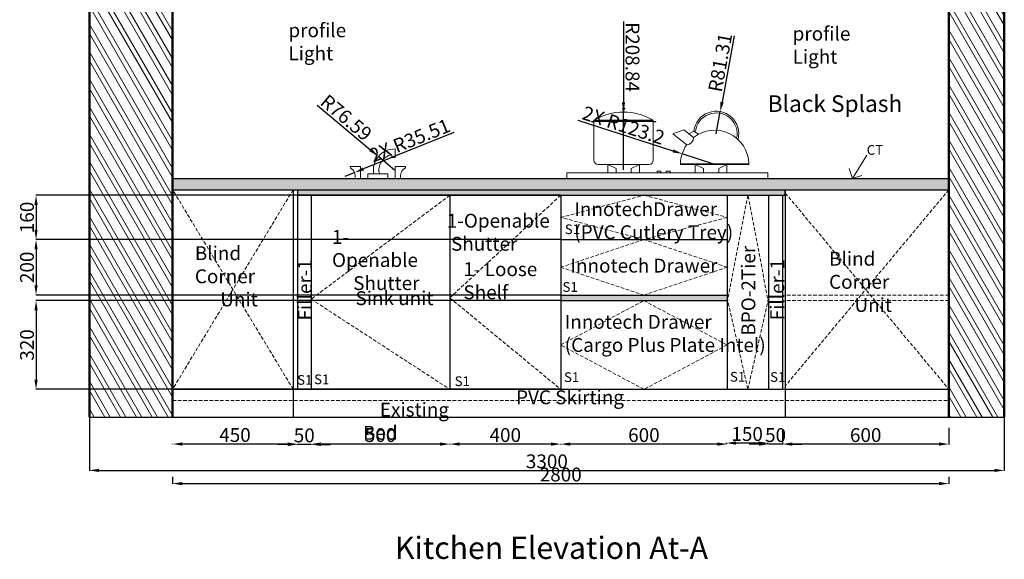
# Model space of a CAD drawing. Units: millimetres. Extents: x 407065 to 421840, y 1168257 to 1177792.
# Tile 12 of 17: x 412177 to 415729, y 1173613 to 1175560. Entities that reach past the tile are written whole.
import ezdxf

# ---------------------------------------------------------------- set-up
doc = ezdxf.new("R2010")
doc.units = ezdxf.units.MM
doc.linetypes.add('DASHED', pattern=[19.05, 12.7, -6.35])
for name, color, linetype, lineweight in [('A-ANNO-DIMS', 6, 'Continuous', 18), ('A-ANNO-SYMB', 6, 'Continuous', 18), ('A-ANNO-TEXT', 30, 'Continuous', 18), ('A-EQPM', 8, 'Continuous', 18), ('A-FURN', 3, 'Continuous', 25), ('A-FURN-HIDN', 7, 'DASHED', 18), ('A-FURN-PATT', 252, 'Continuous', 13), ('A-WALL', 7, 'Continuous', 50), ('A-WALL-PATT', 8, 'Continuous', 13)]:
    doc.layers.add(name, color=color, linetype=linetype, lineweight=lineweight)
doc.styles.get("Standard").update_dxf_attribs({"font": 'arial.ttf'})
doc.dimstyles.new('ISO-25', dxfattribs={"dimtxt": 50, "dimasz": 35, "dimexe": 1.25, "dimexo": 0.625, "dimtad": 1, "dimdec": 1, "dimtxsty": 'Standard', "dimcen": 35, "dimadec": 0, "dimazin": 0, "dimtfac": 1, "dimtdec": 1, "dimtmove": 0, "dimatfit": 3, "dimfxl": 1, "dimarcsym": 0})
pattern_1 = [(120, (-2714.86, -161.38), (-42.8942382, -24.765), []), (120, (-2708.816, -138.83), (-42.8942382, -24.765), [])]

# ---------------------------------------------------------------- blocks, each defined once
blk = doc.blocks.new('*D72')
at = {"layer": 'A-ANNO-DIMS', "color": 0, "lineweight": -2, "transparency": 16777216}
for p, q in [((415528.5, 1174087.5), (415528.5, 1174027.5)), ((414928.5, 1174080.3), (414928.5, 1174027.5)), ((415493.5, 1174028.8), (414963.5, 1174028.8))]:
    blk.add_line(p, q, dxfattribs=at)
at = {"layer": 'A-ANNO-DIMS', "color": 0, "transparency": 16777216}
for points in [[(414963.5, 1174034.6), (414963.5, 1174022.9), (414928.5, 1174028.8)], [(415493.5, 1174034.6), (415493.5, 1174022.9), (415528.5, 1174028.8)]]:
    blk.add_solid(points, dxfattribs=at)
at = {"layer": 'Defpoints', "color": 0, "transparency": 16777216}
for p in [(415528.5, 1174088.1), (414928.5, 1174080.9), (414928.5, 1174028.8)]:
    blk.add_point(p, dxfattribs=at)
at = {"layer": 'A-ANNO-DIMS', "color": 0, "transparency": 16777216, "insert": (415228.5, 1174054.9), "char_height": 50, "attachment_point": 5}
blk.add_mtext('600', dxfattribs=at)
blk = doc.blocks.new('*D73')
at = {"layer": 'A-ANNO-DIMS', "color": 0, "lineweight": -2, "transparency": 16777216}
for p, q in [((414843.5, 1174028.8), (414808.5, 1174028.8)), ((414878.5, 1174029.4), (414878.5, 1174030)), ((414928.5, 1174028.8), (414878.5, 1174028.8)), ((414928.5, 1174029.4), (414928.5, 1174030)), ((414963.5, 1174028.8), (414998.5, 1174028.8))]:
    blk.add_line(p, q, dxfattribs=at)
at = {"layer": 'A-ANNO-DIMS', "color": 0, "transparency": 16777216}
for points in [[(414843.5, 1174034.6), (414843.5, 1174022.9), (414878.5, 1174028.8)], [(414963.5, 1174034.6), (414963.5, 1174022.9), (414928.5, 1174028.8)]]:
    blk.add_solid(points, dxfattribs=at)
at = {"layer": 'Defpoints', "color": 0, "transparency": 16777216}
for p in [(414878.5, 1174028.8), (414878.5, 1174028.8), (414928.5, 1174028.8)]:
    blk.add_point(p, dxfattribs=at)
at = {"layer": 'A-ANNO-DIMS', "color": 0, "transparency": 16777216, "insert": (414903.5, 1174054.9), "char_height": 50, "attachment_point": 5}
blk.add_mtext('50', dxfattribs=at)
blk = doc.blocks.new('*D74')
at = {"layer": 'A-ANNO-DIMS', "color": 0, "lineweight": -2, "transparency": 16777216}
for p, q in [((414725.9, 1174029.4), (414725.9, 1174033.8)), ((414840.9, 1174032.5), (414760.9, 1174032.5)), ((414875.9, 1174029.4), (414875.9, 1174033.8))]:
    blk.add_line(p, q, dxfattribs=at)
at = {"layer": 'A-ANNO-DIMS', "color": 0, "transparency": 16777216}
for points in [[(414760.9, 1174038.4), (414760.9, 1174026.7), (414725.9, 1174032.5)], [(414840.9, 1174038.4), (414840.9, 1174026.7), (414875.9, 1174032.5)]]:
    blk.add_solid(points, dxfattribs=at)
at = {"layer": 'Defpoints', "color": 0, "transparency": 16777216}
for p in [(414725.9, 1174032.5), (414725.9, 1174028.8), (414875.9, 1174028.8)]:
    blk.add_point(p, dxfattribs=at)
at = {"layer": 'A-ANNO-DIMS', "color": 0, "transparency": 16777216, "insert": (414800.9, 1174058.7), "char_height": 50, "attachment_point": 5}
blk.add_mtext('150', dxfattribs=at)
blk = doc.blocks.new('*D75')
at = {"layer": 'A-ANNO-DIMS', "color": 0, "lineweight": -2, "transparency": 16777216}
for p, q in [((414128.5, 1174029.4), (414128.5, 1174030)), ((414693.5, 1174028.8), (414163.5, 1174028.8)), ((414728.5, 1174029.4), (414728.5, 1174030))]:
    blk.add_line(p, q, dxfattribs=at)
at = {"layer": 'A-ANNO-DIMS', "color": 0, "transparency": 16777216}
for points in [[(414163.5, 1174034.6), (414163.5, 1174022.9), (414128.5, 1174028.8)], [(414693.5, 1174034.6), (414693.5, 1174022.9), (414728.5, 1174028.8)]]:
    blk.add_solid(points, dxfattribs=at)
at = {"layer": 'Defpoints', "color": 0, "transparency": 16777216}
for p in [(414128.5, 1174028.8), (414128.5, 1174028.8), (414728.5, 1174028.8)]:
    blk.add_point(p, dxfattribs=at)
at = {"layer": 'A-ANNO-DIMS', "color": 0, "transparency": 16777216, "insert": (414428.5, 1174054.9), "char_height": 50, "attachment_point": 5}
blk.add_mtext('600', dxfattribs=at)
blk = doc.blocks.new('*D76')
at = {"layer": 'A-ANNO-DIMS', "color": 0, "lineweight": -2, "transparency": 16777216}
for p, q in [((413728.5, 1174029.4), (413728.5, 1174027.5)), ((414093.5, 1174028.8), (413763.5, 1174028.8)), ((414128.5, 1174029.4), (414128.5, 1174027.5))]:
    blk.add_line(p, q, dxfattribs=at)
at = {"layer": 'A-ANNO-DIMS', "color": 0, "transparency": 16777216}
for points in [[(413763.5, 1174034.6), (413763.5, 1174022.9), (413728.5, 1174028.8)], [(414093.5, 1174034.6), (414093.5, 1174022.9), (414128.5, 1174028.8)]]:
    blk.add_solid(points, dxfattribs=at)
at = {"layer": 'Defpoints', "color": 0, "transparency": 16777216}
for p in [(413728.5, 1174030), (413728.5, 1174028.8), (414128.5, 1174030)]:
    blk.add_point(p, dxfattribs=at)
at = {"layer": 'A-ANNO-DIMS', "color": 0, "transparency": 16777216, "insert": (413928.5, 1174054.9), "char_height": 50, "attachment_point": 5}
blk.add_mtext('400', dxfattribs=at)
blk = doc.blocks.new('*D77')
at = {"layer": 'A-ANNO-DIMS', "color": 0, "lineweight": -2, "transparency": 16777216}
for p, q in [((413228.5, 1174028.1), (413228.5, 1174030)), ((413693.5, 1174028.8), (413263.5, 1174028.8)), ((413728.5, 1174028.1), (413728.5, 1174030))]:
    blk.add_line(p, q, dxfattribs=at)
at = {"layer": 'A-ANNO-DIMS', "color": 0, "transparency": 16777216}
for points in [[(413263.5, 1174034.6), (413263.5, 1174022.9), (413228.5, 1174028.8)], [(413693.5, 1174034.6), (413693.5, 1174022.9), (413728.5, 1174028.8)]]:
    blk.add_solid(points, dxfattribs=at)
at = {"layer": 'Defpoints', "color": 0, "transparency": 16777216}
for p in [(413228.5, 1174028.8), (413228.5, 1174027.5), (413728.5, 1174027.5)]:
    blk.add_point(p, dxfattribs=at)
at = {"layer": 'A-ANNO-DIMS', "color": 0, "transparency": 16777216, "insert": (413478.5, 1174054.9), "char_height": 50, "attachment_point": 5}
blk.add_mtext('500', dxfattribs=at)
blk = doc.blocks.new('*D78')
at = {"layer": 'A-ANNO-DIMS', "color": 0, "lineweight": -2, "transparency": 16777216}
for p, q in [((413143.5, 1174027.5), (413108.5, 1174027.5)), ((413178.5, 1174028.1), (413178.5, 1174028.8)), ((413228.5, 1174027.5), (413178.5, 1174027.5)), ((413228.5, 1174028.1), (413228.5, 1174028.8)), ((413263.5, 1174027.5), (413298.5, 1174027.5))]:
    blk.add_line(p, q, dxfattribs=at)
at = {"layer": 'A-ANNO-DIMS', "color": 0, "transparency": 16777216}
for points in [[(413143.5, 1174033.4), (413143.5, 1174021.7), (413178.5, 1174027.5)], [(413263.5, 1174033.4), (413263.5, 1174021.7), (413228.5, 1174027.5)]]:
    blk.add_solid(points, dxfattribs=at)
at = {"layer": 'Defpoints', "color": 0, "transparency": 16777216}
for p in [(413178.5, 1174027.5), (413178.5, 1174027.5), (413228.5, 1174027.5)]:
    blk.add_point(p, dxfattribs=at)
at = {"layer": 'A-ANNO-DIMS', "color": 0, "transparency": 16777216, "insert": (413203.5, 1174053.7), "char_height": 50, "attachment_point": 5}
blk.add_mtext('50', dxfattribs=at)
blk = doc.blocks.new('*D79')
at = {"layer": 'A-ANNO-DIMS', "color": 0, "lineweight": -2, "transparency": 16777216}
for p, q in [((412728.5, 1174028.1), (412728.5, 1174030.2)), ((413143.5, 1174028.9), (412763.5, 1174028.9)), ((413178.5, 1174028.1), (413178.5, 1174030.2))]:
    blk.add_line(p, q, dxfattribs=at)
at = {"layer": 'A-ANNO-DIMS', "color": 0, "transparency": 16777216}
for points in [[(412763.5, 1174034.8), (412763.5, 1174023.1), (412728.5, 1174028.9)], [(413143.5, 1174034.8), (413143.5, 1174023.1), (413178.5, 1174028.9)]]:
    blk.add_solid(points, dxfattribs=at)
at = {"layer": 'Defpoints', "color": 0, "transparency": 16777216}
for p in [(412728.5, 1174028.9), (412728.5, 1174027.5), (413178.5, 1174027.5)]:
    blk.add_point(p, dxfattribs=at)
at = {"layer": 'A-ANNO-DIMS', "color": 0, "transparency": 16777216, "insert": (412953.5, 1174055.1), "char_height": 50, "attachment_point": 5}
blk.add_mtext('450', dxfattribs=at)
blk = doc.blocks.new('*D80')
at = {"layer": 'A-ANNO-DIMS', "color": 0, "lineweight": -2, "transparency": 16777216}
for p, q in [((412728.5, 1173911), (412728.5, 1173885)), ((415528.5, 1173911), (415528.5, 1173885)), ((412763.5, 1173886.3), (415493.5, 1173886.3))]:
    blk.add_line(p, q, dxfattribs=at)
at = {"layer": 'A-ANNO-DIMS', "color": 0, "transparency": 16777216}
for points in [[(412763.5, 1173892.1), (412763.5, 1173880.5), (412728.5, 1173886.3)], [(415493.5, 1173892.1), (415493.5, 1173880.5), (415528.5, 1173886.3)]]:
    blk.add_solid(points, dxfattribs=at)
at = {"layer": 'Defpoints', "color": 0, "transparency": 16777216}
for p in [(412728.5, 1173911.6), (415528.5, 1173911.6), (415528.5, 1173886.3)]:
    blk.add_point(p, dxfattribs=at)
at = {"layer": 'A-ANNO-DIMS', "color": 0, "transparency": 16777216, "insert": (414128.5, 1173912.4), "char_height": 50, "attachment_point": 5}
blk.add_mtext('2800', dxfattribs=at)
blk = doc.blocks.new('*D193')
at = {"layer": 'A-ANNO-DIMS', "color": 0, "lineweight": -2, "transparency": 16777216}
for p, q in [((412428.5, 1174125.8), (412428.5, 1173932.7)), ((415728.5, 1174125.8), (415728.5, 1173932.7)), ((412463.5, 1173933.9), (415693.5, 1173933.9))]:
    blk.add_line(p, q, dxfattribs=at)
at = {"layer": 'A-ANNO-DIMS', "color": 0, "transparency": 16777216}
for points in [[(412463.5, 1173939.7), (412463.5, 1173928.1), (412428.5, 1173933.9)], [(415693.5, 1173939.7), (415693.5, 1173928.1), (415728.5, 1173933.9)]]:
    blk.add_solid(points, dxfattribs=at)
at = {"layer": 'Defpoints', "color": 0, "transparency": 16777216}
for p in [(412428.5, 1174126.4), (415728.5, 1174126.4), (415728.5, 1173933.9)]:
    blk.add_point(p, dxfattribs=at)
at = {"layer": 'A-ANNO-DIMS', "color": 0, "transparency": 16777216, "insert": (414078.5, 1173960.1), "char_height": 50, "attachment_point": 5}
blk.add_mtext('3300', dxfattribs=at)
blk = doc.blocks.new('*D197')
at = {"layer": 'A-ANNO-DIMS', "color": 0, "lineweight": -2, "transparency": 16777216}
for p, q in [((414127.9, 1174926.4), (412234.8, 1174926.4)), ((412236, 1174891.4), (412236, 1174801.4)), ((414127.9, 1174766.4), (412234.8, 1174766.4))]:
    blk.add_line(p, q, dxfattribs=at)
at = {"layer": 'A-ANNO-DIMS', "color": 0, "transparency": 16777216}
for points in [[(412230.2, 1174891.4), (412241.8, 1174891.4), (412236, 1174926.4)], [(412230.2, 1174801.4), (412241.8, 1174801.4), (412236, 1174766.4)]]:
    blk.add_solid(points, dxfattribs=at)
at = {"layer": 'Defpoints', "color": 0, "transparency": 16777216}
for p in [(414128.5, 1174926.4), (412236, 1174766.4), (414128.5, 1174766.4)]:
    blk.add_point(p, dxfattribs=at)
at = {"layer": 'A-ANNO-DIMS', "color": 0, "transparency": 16777216, "insert": (412209.8, 1174846.4), "char_height": 50, "attachment_point": 5, "rotation": 90}
blk.add_mtext('160', dxfattribs=at)
blk = doc.blocks.new('*D198')
at = {"layer": 'A-ANNO-DIMS', "color": 0, "lineweight": -2, "transparency": 16777216}
for p, q in [((414127.9, 1174766.4), (412234.8, 1174766.4)), ((412236, 1174731.4), (412236, 1174601.4)), ((414127.9, 1174566.4), (412234.8, 1174566.4))]:
    blk.add_line(p, q, dxfattribs=at)
at = {"layer": 'A-ANNO-DIMS', "color": 0, "transparency": 16777216}
for points in [[(412230.2, 1174731.4), (412241.8, 1174731.4), (412236, 1174766.4)], [(412230.2, 1174601.4), (412241.8, 1174601.4), (412236, 1174566.4)]]:
    blk.add_solid(points, dxfattribs=at)
at = {"layer": 'Defpoints', "color": 0, "transparency": 16777216}
for p in [(414128.5, 1174766.4), (412236, 1174566.4), (414128.5, 1174566.4)]:
    blk.add_point(p, dxfattribs=at)
at = {"layer": 'A-ANNO-DIMS', "color": 0, "transparency": 16777216, "insert": (412209.8, 1174666.4), "char_height": 50, "attachment_point": 5, "rotation": 90}
blk.add_mtext('200', dxfattribs=at)
blk = doc.blocks.new('*D199')
at = {"layer": 'A-ANNO-DIMS', "color": 0, "lineweight": -2, "transparency": 16777216}
for p, q in [((414127.9, 1174546.4), (412234.8, 1174546.4)), ((412236, 1174511.4), (412236, 1174261.4)), ((414127.9, 1174226.4), (412234.8, 1174226.4))]:
    blk.add_line(p, q, dxfattribs=at)
at = {"layer": 'A-ANNO-DIMS', "color": 0, "transparency": 16777216}
for points in [[(412230.2, 1174511.4), (412241.8, 1174511.4), (412236, 1174546.4)], [(412230.2, 1174261.4), (412241.8, 1174261.4), (412236, 1174226.4)]]:
    blk.add_solid(points, dxfattribs=at)
at = {"layer": 'Defpoints', "color": 0, "transparency": 16777216}
for p in [(414128.5, 1174546.4), (412236, 1174226.4), (414128.5, 1174226.4)]:
    blk.add_point(p, dxfattribs=at)
at = {"layer": 'A-ANNO-DIMS', "color": 0, "transparency": 16777216, "insert": (412209.8, 1174386.4), "char_height": 50, "attachment_point": 5, "rotation": 90}
blk.add_mtext('320', dxfattribs=at)
blk = doc.blocks.new('*D234')
at = {"layer": 'A-ANNO-DIMS', "color": 0, "lineweight": -2, "transparency": 16777216}
for p, q in [((414354.6, 1175552.9), (414355, 1175261.4)), ((414355.2, 1175017.6), (414355, 1175226.4))]:
    blk.add_line(p, q, dxfattribs=at)
at = {"layer": 'A-ANNO-DIMS', "color": 0, "transparency": 16777216}
blk.add_solid([(414360.8, 1175261.4), (414349.1, 1175261.4), (414355, 1175226.4)], dxfattribs=at)
at = {"layer": 'Defpoints', "color": 0, "transparency": 16777216}
for p in [(414355, 1175226.4), (414355.2, 1175017.6)]:
    blk.add_point(p, dxfattribs=at)
at = {"layer": 'A-ANNO-DIMS', "color": 0, "transparency": 16777216, "insert": (414380.9, 1175424.7), "char_height": 50, "attachment_point": 5, "rotation": 270.0628}
blk.add_mtext('R208.84', dxfattribs=at)
blk = doc.blocks.new('*D235')
at = {"layer": 'A-ANNO-DIMS', "color": 0, "lineweight": -2, "transparency": 16777216}
for p, q in [((414190.2, 1175197.6), (414533.3, 1175086.6)), ((414683.8, 1175037.9), (414566.6, 1175075.8))]:
    blk.add_line(p, q, dxfattribs=at)
at = {"layer": 'A-ANNO-DIMS', "color": 0, "transparency": 16777216}
blk.add_solid([(414535.1, 1175092.1), (414531.5, 1175081), (414566.6, 1175075.8)], dxfattribs=at)
at = {"layer": 'Defpoints', "color": 0, "transparency": 16777216}
for p in [(414566.6, 1175075.8), (414683.8, 1175037.9)]:
    blk.add_point(p, dxfattribs=at)
at = {"layer": 'A-ANNO-DIMS', "color": 0, "transparency": 16777216, "insert": (414353.1, 1175172.4), "char_height": 50, "attachment_point": 5, "rotation": 342.069}
blk.add_mtext('2X R123.2', dxfattribs=at)
blk = doc.blocks.new('*D236')
at = {"layer": 'A-ANNO-DIMS', "color": 0, "lineweight": -2, "transparency": 16777216}
for p, q in [((414754.6, 1175501.6), (414710.5, 1175262.4)), ((414689.5, 1175148.1), (414704.2, 1175228))]:
    blk.add_line(p, q, dxfattribs=at)
at = {"layer": 'A-ANNO-DIMS', "color": 0, "transparency": 16777216}
blk.add_solid([(414704.8, 1175263.5), (414716.3, 1175261.4), (414704.2, 1175228)], dxfattribs=at)
at = {"layer": 'Defpoints', "color": 0, "transparency": 16777216}
for p in [(414704.2, 1175228), (414689.5, 1175148.1)]:
    blk.add_point(p, dxfattribs=at)
at = {"layer": 'A-ANNO-DIMS', "color": 0, "transparency": 16777216, "insert": (414710, 1175404), "char_height": 50, "attachment_point": 5, "rotation": 79.5666}
blk.add_mtext('R81.31', dxfattribs=at)
blk = doc.blocks.new('*D237')
at = {"layer": 'A-ANNO-DIMS', "color": 0, "lineweight": -2, "transparency": 16777216}
for p, q in [((413250.5, 1175251.6), (413444, 1175088.7)), ((413529.4, 1175016.9), (413470.8, 1175066.2))]:
    blk.add_line(p, q, dxfattribs=at)
at = {"layer": 'A-ANNO-DIMS', "color": 0, "transparency": 16777216}
blk.add_solid([(413447.8, 1175093.2), (413440.2, 1175084.3), (413470.8, 1175066.2)], dxfattribs=at)
at = {"layer": 'Defpoints', "color": 0, "transparency": 16777216}
for p in [(413470.8, 1175066.2), (413529.4, 1175016.9)]:
    blk.add_point(p, dxfattribs=at)
at = {"layer": 'A-ANNO-DIMS', "color": 0, "transparency": 16777216, "insert": (413350.7, 1175201.5), "char_height": 50, "attachment_point": 5, "rotation": 319.9077}
blk.add_mtext('R76.59', dxfattribs=at)
blk = doc.blocks.new('*D238')
at = {"layer": 'A-ANNO-DIMS', "color": 0, "lineweight": -2, "transparency": 16777216}
for p, q in [((413742.7, 1175153), (413416.9, 1175021.3)), ((413351.5, 1174994.9), (413384.4, 1175008.2))]:
    blk.add_line(p, q, dxfattribs=at)
at = {"layer": 'A-ANNO-DIMS', "color": 0, "transparency": 16777216}
blk.add_solid([(413414.7, 1175026.7), (413419.1, 1175015.9), (413384.4, 1175008.2)], dxfattribs=at)
at = {"layer": 'Defpoints', "color": 0, "transparency": 16777216}
for p in [(413384.4, 1175008.2), (413351.5, 1174994.9)]:
    blk.add_point(p, dxfattribs=at)
at = {"layer": 'A-ANNO-DIMS', "color": 0, "transparency": 16777216, "insert": (413586.2, 1175118), "char_height": 50, "attachment_point": 5, "rotation": 22.0142}
blk.add_mtext('2X R35.51', dxfattribs=at)

msp = doc.modelspace()

# ---------------------------------------------------------------- hatches: boundary and pattern name
at = {"layer": 'A-FURN-PATT'}
h = msp.add_hatch(dxfattribs=at)
h.set_pattern_fill('AR-CONC', color=256, scale=0.08)
h.set_pattern_definition([(50, (-2714.86, -161.382), (14.57477352, -1.27512684), [1.524, -16.764]), (355, (-2714.86, -161.382), (-2.81947371, 15.28454762), [1.2192, -13.41124673]), (100.4514447, (-2713.645, -161.488), (11.75529977, 14.00942015), [1.2952007, -14.24721957]), (46.1842, (-2714.86, -157.318), (21.68632327, -3.36338623), [2.286, -25.146]), (96.6355576, (-2713.052, -157.598), (18.99233072, 19.79408997), [1.94280185, -21.37084865]), (351.1841512, (-2714.86, -157.318), (18.99233073, 19.79408997), [1.82879737, -20.11677855]), (21, (-2712.827, -158.334), (12.1291513, -8.18121585), [1.524, -16.764]), (326, (-2712.827, -158.334), (4.94416227, 14.73503729), [1.2192, -13.4112]), (71.451445, (-2711.817, -159.016), (17.07331354, 6.55382151), [1.2952007, -14.247195]), (37.5, (-2714.8595, -161.382), (0.24708826, 6.76440311), [0, -13.24864, 0, -13.6144, 0, -13.462]), (7.5, (-2714.8595, -161.382), (5.345573, 8.014445985), [0, -7.76224, 0, -12.94384, 0, -5.1308]), (327.5, (-2719.391, -161.382), (10.847247613, -0.45829952), [0, -5.08, 0, -15.8496, 0, -21.0312]), (317.5, (-2721.423, -161.382), (11.85033451, 2.03411928), [0, -6.604, 0, -10.52576, 0, -14.9352])])
h.paths.add_polyline_path([(415528.5012, 1174986.413), (412728.5012, 1174986.413), (412728.5012, 1174946.413), (415528.5012, 1174946.413)])
h = msp.add_hatch(color=256, dxfattribs=at)
h.dxf.hatch_style = 1
h.paths.add_polyline_path([(414938.5012, 1174946.413), (413178.5012, 1174946.413), (413178.5012, 1174926.413), (414938.5012, 1174926.413)])
h = msp.add_hatch(color=256, dxfattribs=at)
h.dxf.hatch_style = 1
h.paths.add_polyline_path([(414728.5012, 1174566.413), (414128.5012, 1174566.413), (414128.5012, 1174546.413), (414728.5012, 1174546.413)])
at = {"layer": 'A-WALL-PATT'}
h = msp.add_hatch(dxfattribs=at)
h.set_pattern_fill('ANSI32', color=256, scale=5.2, angle=75)
h.set_pattern_definition(pattern_1)
h.paths.add_polyline_path([(412728.5012, 1176976.413), (412428.5012, 1176976.413), (412428.5012, 1174126.413), (412728.5012, 1174126.413)])
h = msp.add_hatch(dxfattribs=at)
h.set_pattern_fill('ANSI32', color=256, scale=5.2, angle=75)
h.set_pattern_definition(pattern_1)
h.paths.add_polyline_path([(415728.5012, 1176976.413), (415528.5012, 1176976.413), (415528.5012, 1174126.413), (415728.5012, 1174126.413)])

# ---------------------------------------------------------------- linework, layer by layer
at = {"layer": 'A-ANNO-SYMB'}
for p, q in [((415232.2383, 1175071.1078), (415180.4443, 1174986.413)), ((415180.4443, 1174986.413), (415168.3118, 1175023.0386)), ((415180.4443, 1174986.413), (415215.0859, 1174997.8883))]:
    msp.add_line(p, q, dxfattribs=at)
at = {"layer": 'A-EQPM'}
for p, q in [((414351.0049, 1175240.2526), (414359.4523, 1175240.2526)), ((414351.0049, 1175240.2526), (414359.4523, 1175240.2526)), ((414351.0049, 1175240.2526), (414351.0049, 1175239.2526)), ((414351.0049, 1175240.1526), (414359.4523, 1175240.1526)), ((414351.0049, 1175240.0526), (414359.4523, 1175240.0526)), ((414351.0049, 1175239.6526), (414359.4523, 1175239.6526)), ((414351.0049, 1175239.5526), (414359.4523, 1175239.5526)), ((414351.0049, 1175239.4526), (414359.4523, 1175239.4526)), ((414351.0049, 1175239.3526), (414359.4523, 1175239.3526)), ((414351.0049, 1175239.2526), (414359.4523, 1175239.2526)), ((414359.4523, 1175240.2526), (414359.4523, 1175239.2526)), ((414243.6848, 1175192.7549), (414243.6848, 1175191.0638)), ((414462.513, 1175196.7549), (414247.9443, 1175196.7549)), ((414247.9443, 1175192.7549), (414247.9443, 1175196.7549)), ((414462.513, 1175194.7549), (414247.9443, 1175194.7549)), ((414247.9443, 1175052.843), (414247.9443, 1175192.7549)), ((414462.513, 1175192.7549), (414247.9443, 1175192.7549)), ((414462.513, 1175192.7549), (414462.513, 1175196.7549)), ((414462.513, 1175052.843), (414462.513, 1175192.7549)), ((414466.7725, 1175192.7549), (414466.7725, 1175191.0638)), ((414533.1417, 1175147.655), (414573.015, 1175161.9682)), ((414607.6829, 1175134.7682), (414573.015, 1175161.9682)), ((414590.3489, 1175148.3682), (414608.7664, 1175158.0185)), ((414608.7664, 1175158.0185), (414625.4451, 1175146.3939)), ((414582.9081, 1175108.6091), (414533.1417, 1175147.655)), ((413531.1651, 1175062.4704), (413531.1651, 1175093.4358)), ((413518.8807, 1175072.4781), (413518.8807, 1175062.4704)), ((413518.8807, 1175062.4704), (413531.1651, 1175062.4704)), ((413406.3058, 1175030.3743), (413369.5761, 1175029.7999)), ((413369.5761, 1175029.7999), (413369.6513, 1175025.3894)), ((413406.3058, 1174986.413), (413406.3058, 1175030.3743)), ((413531.3771, 1174986.413), (413531.3771, 1175030.3743)), ((413531.3771, 1175030.3743), (413568.1068, 1175029.7999)), ((413568.1068, 1175029.7999), (413568.0316, 1175025.3894)), ((414263.0542, 1175037.7331), (414447.4031, 1175037.7331)), ((414560.6069, 1175040.1331), (414806.9496, 1175040.1331)), ((414560.6069, 1175040.1331), (414560.6069, 1175037.7331)), ((414560.6069, 1175039.1331), (414806.9496, 1175039.1331)), ((414560.6069, 1175038.1331), (414806.9496, 1175038.1331)), ((414560.6069, 1175038.0331), (414806.9496, 1175038.0331)), ((414560.6069, 1175037.9331), (414806.9496, 1175037.9331)), ((414560.6069, 1175037.8331), (414806.9496, 1175037.8331)), ((414560.6069, 1175037.7331), (414806.9496, 1175037.7331)), ((414806.9496, 1175040.1331), (414806.9934, 1175037.7331))]:
    msp.add_line(p, q, dxfattribs=at)
for points in [[(414247.9443, 1175192.7549), (414239.4253, 1175192.7549), (414239.4253, 1175191.0638), (414247.9443, 1175191.0638)], [(414462.513, 1175192.7549), (414471.032, 1175192.7549), (414471.032, 1175191.0638), (414462.513, 1175191.0638)], [(414150.6311, 1174986.413), (414876.1267, 1174986.413), (414876.1267, 1175007.625), (414150.6311, 1175007.625)], [(414475.9973, 1175007.625), (414489.5466, 1175007.625), (414489.5466, 1175013.6244), (414475.9973, 1175013.6244)], [(414509.0351, 1175007.625), (414522.7807, 1175007.625), (414522.7807, 1175013.6244), (414509.0351, 1175013.6244)], [(413432.3984, 1174986.413), (413505.2845, 1174986.413), (413505.2845, 1175003.1756), (413432.3984, 1175003.1756)]]:
    msp.add_lwpolyline(points, close=True, dxfattribs=at)
for points in [[(414298.7174, 1175007.625), (414298.7174, 1175037.7331), (414328.3269, 1175022.3298), (414328.3269, 1175007.625)], [(414412.7527, 1175007.625), (414412.7527, 1175037.7331), (414383.1431, 1175022.3298), (414383.1431, 1175007.625)], [(414614.005, 1175007.625), (414614.005, 1175037.7331), (414643.6146, 1175022.3298), (414643.6146, 1175007.625)], [(414728.0404, 1175007.625), (414728.0404, 1175037.7331), (414698.4308, 1175022.3298), (414698.4308, 1175007.625)]]:
    msp.add_lwpolyline(points, dxfattribs=at)
for centre, radius, start, end in [((414355.2286, 1175017.5743), 208.8435, 59.0889452, 120.9110548), ((414342.5448, 1175231.3192), 11.5979, 334.93847, 43.1597348), ((414367.9125, 1175231.3192), 11.5979, 136.8402652, 205.06153), ((414689.4632, 1175148.0546), 81.3096, 345.4563039, 172.9611665), ((414689.4632, 1175148.0546), 75.3096, 347.8187638, 172.9611665), ((414683.7783, 1175037.8882), 123.1918, 1.044154, 128.1481965), ((414581.0723, 1175135.1592), 26.6135, 273.9553578, 359.1582502), ((413529.3609, 1175016.869), 76.588, 88.6501127, 190.2994789), ((414683.7783, 1175037.8882), 123.1918, 144.9654114, 178.955846), ((413529.3609, 1175016.869), 56.588, 100.6729084, 194.0036952), ((414263.0542, 1175052.843), 15.1099, 180, 270), ((414447.4031, 1175052.843), 15.1099, 270, 0), ((413351.5077, 1174994.8629), 35.5114, 346.234566, 59.2744993), ((413586.1752, 1174994.8629), 35.5114, 120.7255007, 193.765434)]:
    msp.add_arc(centre, radius, start, end, dxfattribs=at)
at = {"layer": 'A-FURN'}
for p, q in [((412728.5012, 1174986.413), (415528.5012, 1174986.413)), ((412728.5012, 1174946.413), (415528.5012, 1174946.413)), ((413163.5012, 1174946.413), (413163.5012, 1174126.413)), ((413178.5012, 1174946.413), (413178.5012, 1174226.413)), ((414938.5012, 1174946.413), (414938.5012, 1174126.413)), ((414938.5012, 1174926.413), (414938.5012, 1174946.413)), ((413178.5012, 1174926.413), (414928.5012, 1174926.413)), ((413228.5012, 1174926.413), (413228.5012, 1174226.413)), ((413728.5012, 1174926.413), (413728.5012, 1174226.413)), ((414128.5012, 1174926.413), (414128.5012, 1174226.413)), ((414728.5012, 1174926.413), (414728.5012, 1174226.413)), ((414878.5012, 1174926.413), (414878.5012, 1174226.413)), ((414928.5012, 1174926.413), (414928.5012, 1174226.413)), ((414928.5012, 1174926.413), (414938.5012, 1174926.413)), ((414128.5012, 1174766.413), (414728.5012, 1174766.413)), ((414128.5012, 1174566.413), (414728.5012, 1174566.413)), ((414128.5012, 1174546.413), (414728.5012, 1174546.413)), ((412728.5012, 1174226.413), (415528.5012, 1174226.413)), ((412428.5012, 1174126.413), (415728.5012, 1174126.413))]:
    msp.add_line(p, q, dxfattribs=at)
at = {"layer": 'A-FURN-HIDN'}
for p, q in [((413163.5012, 1174226.413), (412728.5012, 1174946.413)), ((413163.5012, 1174946.413), (412728.5012, 1174226.413)), ((415528.5012, 1174946.413), (414938.5012, 1174238.413)), ((414128.5012, 1174846.413), (414428.5012, 1174926.413)), ((414428.5012, 1174926.413), (414728.5012, 1174846.413)), ((414938.5012, 1174934.413), (415528.5012, 1174226.413)), ((414428.5012, 1174766.413), (414128.5012, 1174846.413)), ((414728.5012, 1174846.413), (414428.5012, 1174766.413)), ((414428.5012, 1174766.413), (414128.5012, 1174666.413)), ((414728.5012, 1174666.413), (414428.5012, 1174766.413)), ((414128.5012, 1174666.413), (414428.5012, 1174566.413)), ((414428.5012, 1174566.413), (414728.5012, 1174666.413)), ((413163.5012, 1174566.413), (412728.5012, 1174566.413)), ((413163.5012, 1174546.413), (412728.5012, 1174546.413)), ((414128.5012, 1174566.413), (413728.5012, 1174566.413)), ((414128.5012, 1174546.413), (413728.5012, 1174546.413)), ((414128.5012, 1174386.413), (414428.5012, 1174546.413)), ((414428.5012, 1174546.413), (414728.5012, 1174386.413)), ((415528.5012, 1174566.413), (414938.5012, 1174566.413)), ((415528.5012, 1174546.413), (414938.5012, 1174546.413)), ((414428.5012, 1174226.413), (414128.5012, 1174386.413)), ((414728.5012, 1174386.413), (414428.5012, 1174226.413)), ((412728.5012, 1174186.413), (415528.5012, 1174186.413))]:
    msp.add_line(p, q, dxfattribs=at)
for points in [[(413728.5012, 1174926.413), (413228.5012, 1174551.4297), (413728.5012, 1174226.413)], [(414128.5012, 1174926.413), (413728.5012, 1174556.413), (414128.5012, 1174226.413)], [(414878.5012, 1174536.413), (414803.5012, 1174926.413), (414728.5012, 1174536.413)], [(414728.5012, 1174556.413), (414803.5012, 1174226.413), (414878.5012, 1174556.413)]]:
    msp.add_lwpolyline(points, dxfattribs=at)
at = {"layer": 'A-WALL'}
for p, q in [((412428.5012, 1176976.413), (412428.5012, 1174126.413)), ((412728.5012, 1176976.413), (412728.5012, 1174126.413)), ((415528.5012, 1176976.413), (415528.5012, 1174126.413)), ((415728.5012, 1176976.413), (415728.5012, 1174126.413))]:
    msp.add_line(p, q, dxfattribs=at)

# ---------------------------------------------------------------- texts
at = {"layer": 'A-ANNO-TEXT', "attachment_point": 1}
for s, width, insert, char_height in [('profile Light', 382.409863, (413146.448, 1175546.492), 50), ('profile Light', 382.409863, (414965.0699, 1175534.3531), 50), ('Black Splash', 506.516765, (414875.0299, 1175286.8389), 60), ('CT', 382.409863, (415232.2383, 1175107.3016), 35), ('InnotechDrawer\\P(PVC Cutlery Trey)', 606.770927, (414177.5815, 1174901.3326), 50), ('     1-Openable\\P      Shutter', 520.083559, (413641.1549, 1174859.5224), 50), ('1- Openable\\P     Shutter', 382.409863, (413303.5103, 1174801.0944), 50), ('S1', 382.409863, (414143.2127, 1174821.305), 35), ('Blind Corner\\P      Unit', 382.409863, (412808.8782, 1174742.3897), 50), ('Blind Corner\\P      Unit', 382.409863, (415096.3782, 1174722.3897), 50), (' Innotech Drawer', 554.50831, (414148.2591, 1174697.4541), 50), ('1- Loose Shelf', 382.409863, (413777.5942, 1174684.6553), 50), ('Sink unit', 382.409863, (413388.2668, 1174580.0755), 50), ('S1', 382.409863, (414134.9367, 1174612.9898), 35), ('Innotech Drawer\\P(Cargo Plus Plate Intel)', 730.841704, (414142.9603, 1174494.6735), 50), ('S1', 382.409863, (413177.825, 1174277.8232), 35), ('S1', 382.409863, (413239.0126, 1174279.8839), 35), ('S1', 382.409863, (413745.9227, 1174273.0119), 35), ('S1', 382.409863, (414140.3355, 1174287.7811), 35), ('S1', 382.409863, (414738.9729, 1174289.0087), 35), ('S1', 382.409863, (414883.7724, 1174288.32), 35), ('    PVC Skirting', 581.712517, (413906.2879, 1174222.6068), 50), ('    Existing Bed', 382.409863, (413415.1834, 1174177.908), 50), ('Kitchen Elevation At-A', 1357.183536, (413530.5499, 1173694.5878), 80)]:
    msp.add_mtext_dynamic_manual_height_columns(s, width=width, gutter_width=12.5, heights=[0], dxfattribs=dict(at, insert=insert, char_height=char_height))
at = {"layer": 'A-ANNO-TEXT', "char_height": 50, "attachment_point": 1, "rotation": 90}
for s, insert in [('  BPO-2Tier', (414780.3802, 1174389.4298)), ('     Filler-1', (413180.4517, 1174398.4786)), ('     Filler-1', (414884.561, 1174398.979))]:
    msp.add_mtext_dynamic_manual_height_columns(s, width=382.409863, gutter_width=12.5, heights=[0], dxfattribs=dict(at, insert=insert))

# ---------------------------------------------------------------- dimensions: what is measured, and where the dimension line sits
at = {"layer": 'A-ANNO-DIMS'}
for center, mpoint, picture, middle in [((414355.2286, 1175017.5743), (414354.9995, 1175226.4177), '*D234', (414380.9357, 1175424.6804)), ((414689.4632, 1175148.0546), (414704.1878, 1175228.0199), '*D236', (414709.9757, 1175403.9676)), ((413529.3609, 1175016.869), (413470.7704, 1175066.1933), '*D237', (413350.7049, 1175201.4575))]:
    dim = msp.add_radius_dim(center=center, mpoint=mpoint, dimstyle='ISO-25', override={"dimdec": 2, "dimlfac": 1, "dimrnd": 0, "dimzin": 0, "dimdsep": 46, "dimlunit": 2}, dxfattribs=at)
    dim.commit()
    dim.dimension.update_dxf_attribs({"geometry": picture, "text_midpoint": middle})
for center, mpoint, override, picture, middle in [((414683.7783, 1175037.8882), (414566.5701, 1175075.8155), {"dimdec": 1, "dimlfac": 1, "dimrnd": 0, "dimzin": 0, "dimdsep": 46, "dimlunit": 2}, '*D235', (414353.134, 1175172.3879)), ((413351.5077, 1174994.8629), (413384.4299, 1175008.1738), {"dimdec": 2, "dimlfac": 1, "dimrnd": 0, "dimzin": 0, "dimdsep": 46, "dimlunit": 2}, '*D238', (413586.2109, 1175117.9855))]:
    dim = msp.add_radius_dim(center=center, mpoint=mpoint, text='2X <>', dimstyle='ISO-25', override=override, dxfattribs=at)
    dim.commit()
    dim.dimension.update_dxf_attribs({"geometry": picture, "text_midpoint": middle})
for base, p1, p2, picture, middle in [((412236.0012, 1174766.413), (414128.5012, 1174926.413), (414128.5012, 1174766.413), '*D197', (412209.8475, 1174846.413)), ((412236.0012, 1174566.413), (414128.5012, 1174766.413), (414128.5012, 1174566.413), '*D198', (412209.8475, 1174666.413)), ((412236.0012, 1174226.413), (414128.5012, 1174546.413), (414128.5012, 1174226.413), '*D199', (412209.8305, 1174386.413))]:
    dim = msp.add_linear_dim(base=base, p1=p1, p2=p2, angle=90, dimstyle='ISO-25', override={"dimdec": 0, "dimlfac": 1, "dimrnd": 0, "dimzin": 0, "dimdsep": 46, "dimlunit": 2}, dxfattribs=at)
    dim.commit()
    dim.dimension.update_dxf_attribs({"geometry": picture, "text_midpoint": middle})
for base, p1, p2, override, picture, middle in [((415728.5012, 1173933.913), (412428.5012, 1174126.413), (415728.5012, 1174126.413), {"dimdec": 0, "dimlfac": 1, "dimrnd": 0, "dimzin": 0, "dimdsep": 46, "dimlunit": 2}, '*D193', (414078.5012, 1173960.0837)), ((412728.5012, 1174028.9237), (413178.5012, 1174027.5189), (412728.5012, 1174027.5189), {"dimclrd": 0, "dimclre": 0, "dimclrt": 0}, '*D79', (412953.5012, 1174055.0774)), ((413228.5012, 1174028.7689), (413728.5012, 1174027.5189), (413228.5012, 1174027.5189), {"dimclrd": 0, "dimclre": 0, "dimclrt": 0}, '*D77', (413478.5012, 1174054.9225)), ((413728.5012, 1174028.7689), (414128.5012, 1174030.0189), (413728.5012, 1174030.0189), {"dimclrd": 0, "dimclre": 0, "dimclrt": 0}, '*D76', (413928.5012, 1174054.9225)), ((414128.5012, 1174028.7689), (414728.5012, 1174028.7689), (414128.5012, 1174028.7689), {"dimclrd": 0, "dimclre": 0, "dimclrt": 0}, '*D75', (414428.5012, 1174054.9225)), ((414725.864, 1174032.5189), (414875.864, 1174028.7689), (414725.864, 1174028.7689), {"dimclrd": 0, "dimclre": 0, "dimclrt": 0}, '*D74', (414800.864, 1174058.6725)), ((414928.5012, 1174028.7689), (415528.5012, 1174088.0868), (414928.5012, 1174080.8933), {"dimclrd": 0, "dimclre": 0, "dimclrt": 0}, '*D72', (415228.5012, 1174054.9225)), ((415528.5012, 1173886.2913), (412728.5012, 1173911.6222), (415528.5012, 1173911.6222), {"dimclrd": 0, "dimclre": 0, "dimclrt": 0}, '*D80', (414128.5012, 1173912.445))]:
    dim = msp.add_linear_dim(base=base, p1=p1, p2=p2, dimstyle='ISO-25', override=override, dxfattribs=at)
    dim.commit()
    dim.dimension.update_dxf_attribs({"geometry": picture, "text_midpoint": middle})
for base, p1, p2, picture, middle in [((413178.5012, 1174027.5189), (413228.5012, 1174027.5189), (413178.5012, 1174027.5189), '*D78', (413203.5012, 1174027.5189)), ((414878.5012, 1174028.7689), (414928.5012, 1174028.7689), (414878.5012, 1174028.7689), '*D73', (414903.5012, 1174028.7689))]:
    dim = msp.add_linear_dim(base=base, p1=p1, p2=p2, dimstyle='ISO-25', override={"dimclrd": 0, "dimclre": 0, "dimclrt": 0}, dxfattribs=at)
    dim.commit()
    dim.dimension.update_dxf_attribs({"geometry": picture, "text_midpoint": middle, "dimtype": 160})

doc.saveas('drawing.dxf')
